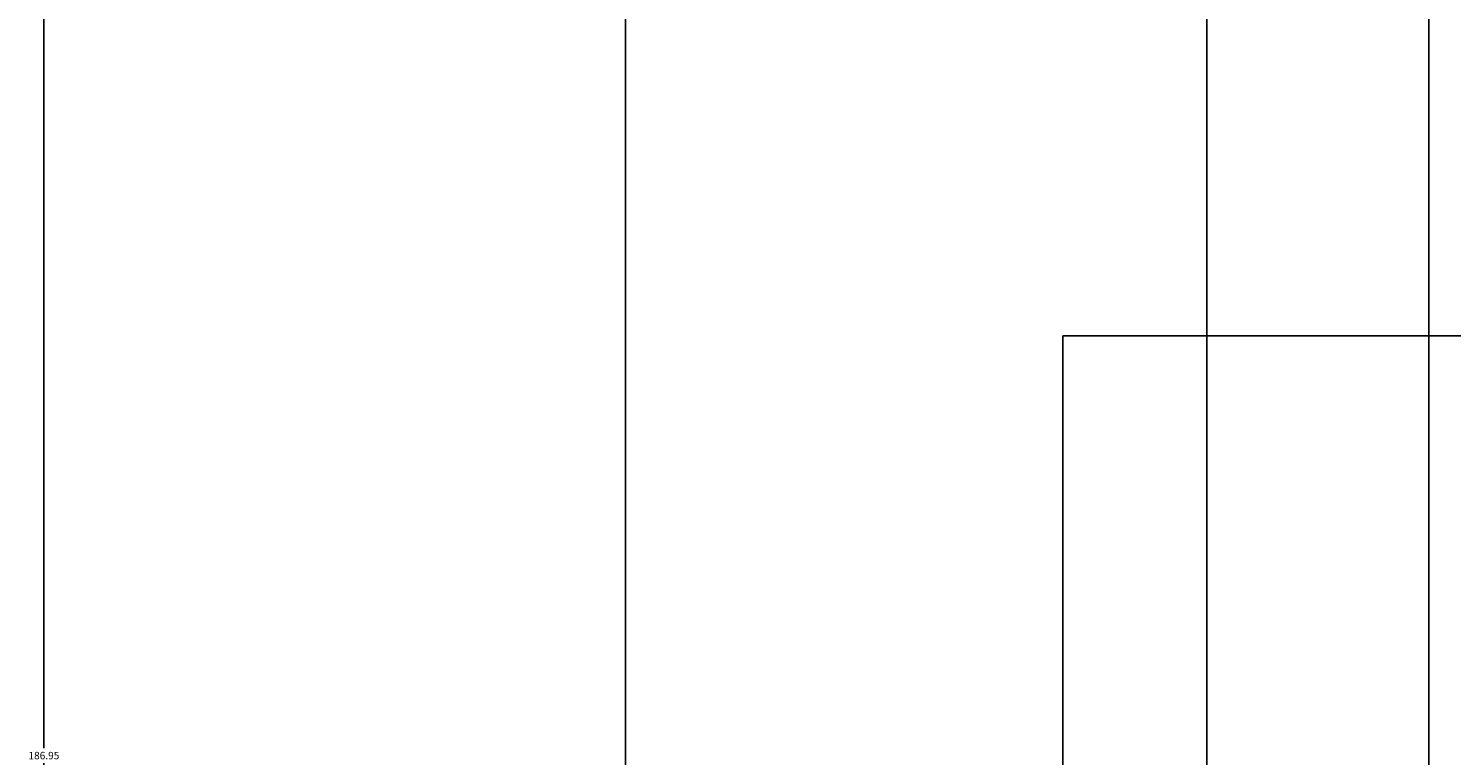
# Model space of a CAD drawing. Units: millimetres. Extents: x -8 to 285, y 5 to 221.
# Tile 10 of 30: x -8 to 27, y 113 to 131. Entities that reach past the tile are written whole.
import ezdxf

# ---------------------------------------------------------------- set-up
doc = ezdxf.new("R2010")
doc.units = ezdxf.units.MM
doc.layers.add('A-ANNO-DIMS', color=2, linetype='Continuous', lineweight=18)
doc.layers.add('E-POWR-DC-NEG', color=3, linetype='Continuous', lineweight=25)
doc.layers.add('E-POWR-DC-POS', color=30, linetype='Continuous', lineweight=25, true_color=0xf26722)
doc.styles.get("Standard").update_dxf_attribs({"font": 'arial.ttf'})
doc.dimstyles.get("Standard").update_dxf_attribs({"dimtxt": 0.18, "dimasz": 0.18, "dimexe": 0.18, "dimexo": 0.0625, "dimgap": 0.09, "dimtad": 0, "dimtih": 1, "dimtoh": 1, "dimdec": 4, "dimzin": 0, "dimdsep": 46, "dimtxsty": 'Standard', "dimcen": 0.09, "dimadec": 0, "dimazin": 0, "dimtfac": 1, "dimtdec": 4, "dimtofl": 0, "dimtmove": 0, "dimatfit": 3, "dimfxl": 1, "dimtolj": 1, "dimtzin": 0, "dimarcsym": 0})

# ---------------------------------------------------------------- blocks, each defined once
blk = doc.blocks.new('*D10')
at = {"layer": 'A-ANNO-DIMS', "color": 0, "lineweight": -2, "transparency": 16777216}
for p, q in [((145.103, 206.457), (-7.608, 206.457)), ((-7.428, 206.277), (-7.428, 113.161)), ((-7.428, 19.682), (-7.428, 112.797)), ((30.453, 19.502), (-7.608, 19.502))]:
    blk.add_line(p, q, dxfattribs=at)
at = {"layer": 'A-ANNO-DIMS', "color": 0, "transparency": 16777216}
for points in [[(-7.458, 206.277), (-7.398, 206.277), (-7.428, 206.457)], [(-7.458, 19.682), (-7.398, 19.682), (-7.428, 19.502)]]:
    blk.add_solid(points, dxfattribs=at)
at = {"layer": 'Defpoints', "color": 0, "transparency": 16777216}
for p in [(-7.428, 206.457), (145.165, 206.457), (30.516, 19.502)]:
    blk.add_point(p, dxfattribs=at)
at = {"layer": 'A-ANNO-DIMS', "color": 0, "transparency": 16777216, "insert": (-7.428, 112.979), "char_height": 0.18, "attachment_point": 5}
blk.add_mtext('\\A1;186.95', dxfattribs=at)
blk = doc.blocks.new('*D19')
at = {"layer": 'A-ANNO-DIMS', "color": 0, "lineweight": -2, "transparency": 16777216}
for p, q in [((6.735, 133.727), (20.952, 133.727)), ((20.772, 133.547), (20.772, 90.056)), ((20.772, 46.201), (20.772, 89.692)), ((6.735, 46.021), (20.952, 46.021))]:
    blk.add_line(p, q, dxfattribs=at)
at = {"layer": 'A-ANNO-DIMS', "color": 0, "transparency": 16777216}
for points in [[(20.742, 133.547), (20.802, 133.547), (20.772, 133.727)], [(20.742, 46.201), (20.802, 46.201), (20.772, 46.021)]]:
    blk.add_solid(points, dxfattribs=at)
at = {"layer": 'Defpoints', "color": 0, "transparency": 16777216}
for p in [(6.672, 133.727), (6.672, 46.021), (20.772, 46.021)]:
    blk.add_point(p, dxfattribs=at)
at = {"layer": 'A-ANNO-DIMS', "color": 0, "transparency": 16777216, "insert": (20.772, 89.874), "char_height": 0.18, "attachment_point": 5}
blk.add_mtext('\\A1;87.7', dxfattribs=at)
blk = doc.blocks.new('*D24')
at = {"layer": 'A-ANNO-DIMS', "color": 0, "lineweight": -2, "transparency": 16777216}
for p, q in [((6.672, 46.084), (6.672, 220.737)), ((6.852, 220.557), (15.959, 220.557)), ((25.975, 220.557), (16.869, 220.557)), ((26.155, 65.791), (26.155, 220.737))]:
    blk.add_line(p, q, dxfattribs=at)
at = {"layer": 'A-ANNO-DIMS', "color": 0, "transparency": 16777216}
for points in [[(6.852, 220.587), (6.852, 220.527), (6.672, 220.557)], [(25.975, 220.587), (25.975, 220.527), (26.155, 220.557)]]:
    blk.add_solid(points, dxfattribs=at)
at = {"layer": 'Defpoints', "color": 0, "transparency": 16777216}
for p in [(26.155, 220.557), (26.155, 65.728), (6.672, 46.021)]:
    blk.add_point(p, dxfattribs=at)
at = {"layer": 'A-ANNO-DIMS', "color": 0, "transparency": 16777216, "insert": (16.414, 220.557), "char_height": 0.18, "attachment_point": 5}
blk.add_mtext('\\A1;19.483', dxfattribs=at)

msp = doc.modelspace()

# ---------------------------------------------------------------- linework, layer by layer
at = {"layer": 'E-POWR-DC-NEG'}
msp.add_lwpolyline([(46.1717, 67.9064), (46.1717, 46.0211), (6.6725, 46.0211), (6.6725, 133.7273), (20.0566, 133.7273), (20.0566, 145.2715)], dxfattribs=at)
at = {"layer": 'E-POWR-DC-POS'}
msp.add_lwpolyline([(74.9801, 145.2715), (74.9801, 123.1618), (17.279, 123.1618), (17.279, 54.6776), (40.1717, 54.6776), (40.1717, 67.9064)], dxfattribs=at)

# ---------------------------------------------------------------- dimensions: what is measured, and where the dimension line sits
at = {"layer": 'A-ANNO-DIMS'}
dim = msp.add_linear_dim(base=(26.1554, 220.5568), p1=(6.6725, 46.0211), p2=(26.1554, 65.7282), dimstyle='Standard', override={"dimdec": 3, "dimlfac": 1, "dimrnd": 0, "dimzin": 0, "dimdsep": 46, "dimlunit": 2}, dxfattribs=at)
dim.commit()
dim.dimension.update_dxf_attribs({"geometry": '*D24', "text_midpoint": (16.4139, 220.5568)})
for base, p1, p2, angle, override, picture, middle in [((-7.4275, 206.4568), (30.516, 19.502), (145.1651, 206.4568), 90, {"dimdec": 2, "dimlfac": 1, "dimrnd": 0, "dimzin": 0, "dimdsep": 46, "dimlunit": 2}, '*D10', (-7.4275, 112.9794)), ((20.7725, 46.0211), (6.6725, 133.7273), (6.6725, 46.0211), 270, {"dimdec": 1, "dimlfac": 1, "dimrnd": 0, "dimzin": 0, "dimdsep": 46, "dimlunit": 2}, '*D19', (20.7725, 89.8742))]:
    dim = msp.add_linear_dim(base=base, p1=p1, p2=p2, angle=angle, dimstyle='Standard', override=override, dxfattribs=at)
    dim.commit()
    dim.dimension.update_dxf_attribs({"geometry": picture, "text_midpoint": middle})

doc.saveas('drawing.dxf')
